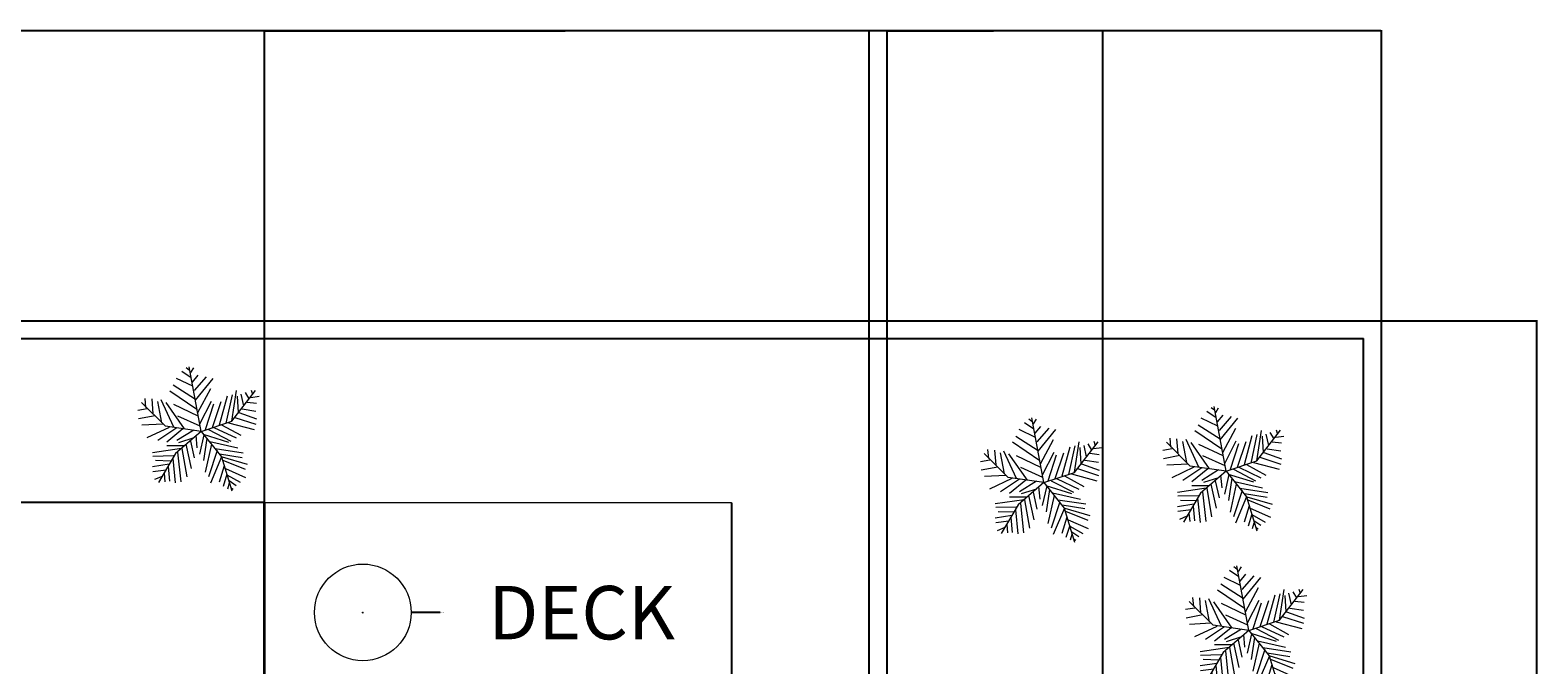
# Model space of a CAD drawing. Units: inches. Extents: x -86 to 773, y -188 to 560.
# Tile 6 of 6: x 392 to 773, y 400 to 560. Entities that reach past the tile are written whole.
import ezdxf

# ---------------------------------------------------------------- set-up
doc = ezdxf.new("R2010")
doc.units = ezdxf.units.IN
doc.header["$MEASUREMENT"] = 0
for name, color, linetype, lineweight in [('A-ANNO-DIMS', 2, 'Continuous', 18), ('A-AREA-IDEN', 7, 'Continuous', 25), ('A-FURN', 8, 'Continuous', 18), ('A-WALL', 7, 'Continuous', 35), ('C-PROP', 7, 'Continuous', 25), ('L-HRDS', 7, 'Continuous', 18), ('L-PLNT-TREE', 8, 'Continuous', 9)]:
    doc.layers.add(name, color=color, linetype=linetype, lineweight=lineweight)
doc.styles.get("Standard").update_dxf_attribs({"font": 'arial.ttf'})
doc.dimstyles.get("Standard").update_dxf_attribs({"dimtxt": 0.18, "dimasz": 0.18, "dimexe": 0.18, "dimexo": 0.0625, "dimgap": 0.09, "dimtad": 0, "dimtih": 1, "dimtoh": 1, "dimdec": 4, "dimzin": 0, "dimdsep": 46, "dimtxsty": 'Standard', "dimcen": 0.09, "dimadec": 0, "dimazin": 0, "dimtfac": 1, "dimtdec": 4, "dimtofl": 0, "dimtmove": 0, "dimatfit": 3, "dimfxl": 1, "dimtolj": 1, "dimtzin": 0, "dimarcsym": 0})

# ---------------------------------------------------------------- blocks, each defined once
blk = doc.blocks.new('Trees - Metric')
for p, q in [((-258.7244, 1362.456), (-332.3336, 1421.4348)), ((0, 0), (-266.7, 1447.8)), ((-231.1146, 1315.2628), (-166.7002, 1421.4348)), ((-129.8956, 713.6638), (-626.7704, 1032.1544)), ((-185.1152, 1008.5578), (-553.1612, 1185.4942)), ((-221.9198, 1197.3052), (-433.5526, 1338.8594)), ((-194.31, 1102.9442), (-65.4812, 1256.284)), ((-148.3106, 914.1968), (118.5418, 1220.9018)), ((-129.8956, 701.8528), (265.7602, 1185.4942)), ((-1234.059, 536.7274), (-1252.4486, 737.2604)), ((-1105.2302, 725.4494), (-1077.6458, 395.1732)), ((-902.8176, 713.6638), (-617.5756, 100.2538)), ((-93.091, 489.5342), (-700.3796, 902.3858)), ((-74.7014, 418.7444), (219.7608, 961.39)), ((-28.6766, 171.0436), (228.9556, 678.2816)), ((412.9786, 147.447), (587.8068, 796.2392)), ((560.197, 182.8292), (698.2206, 819.8358)), ((685.8, 228.6), (1219.2, 914.4)), ((689.0258, 230.0224), (790.2448, 914.1968)), ((808.6344, 784.4282), (827.0494, 418.7444)), ((891.4384, 831.6214), (946.658, 572.1096)), ((983.4626, 867.0036), (1066.2666, 725.4494)), ((1112.2914, 760.8316), (1296.3144, 784.4282)), ((1121.4862, 925.9824), (1149.0706, 831.6214)), ((-1206.4492, 501.3198), (-1418.082, 465.9376)), ((-1031.621, 347.98), (-1399.667, 277.1902)), ((-800.1, 114.3), (-1333.5, 647.7)), ((-976.4268, 666.4706), (-884.4026, 194.6402)), ((-369.1382, 53.086), (-783.1836, 642.874)), ((-617.5756, 607.4918), (-74.7014, 347.98)), ((-525.5514, 347.98), (-28.6766, 123.8504)), ((100.1268, 41.275), (284.1498, 619.2774)), ((256.5654, 88.4682), (449.7832, 666.4706)), ((845.439, 418.7444), (1241.0948, 277.1902)), ((919.0482, 501.3198), (1222.6798, 454.152)), ((1029.462, 654.685), (1241.0948, 631.0884)), ((-847.598, 159.2326), (-1326.0578, 135.636)), ((-718.7946, 88.4682), (-1215.644, -147.447)), ((-543.9664, 76.6572), (-967.2066, -206.4512)), ((0, 0), (-800.1, 114.3)), ((-405.9428, 53.086), (-764.794, -241.8334)), ((0, 0), (-571.5, -495.3)), ((-166.7002, 29.4894), (-543.9664, -206.4512)), ((0, 0), (685.8, 228.6)), ((0, 0), (457.2, -571.5)), ((164.5412, 41.275), (661.416, -218.2368)), ((284.1498, 88.4682), (781.0246, -147.447)), ((458.978, 147.447), (891.4384, -88.4682)), ((615.4166, 194.6402), (1185.8752, 41.275)), ((753.4148, 312.5978), (1222.6798, 159.2326)), ((-387.5278, -324.4088), (-764.794, -324.4088)), ((-166.7002, -147.447), (-507.1618, -253.619)), ((-341.5284, -289.0012), (-221.9198, -831.6214)), ((-240.3094, -218.2368), (-157.5054, -595.7062)), ((-120.7008, -88.4682), (-93.091, -371.5766)), ((63.3222, -76.6826), (-37.8714, -513.1308)), ((44.9326, -64.897), (615.4166, -241.8334)), ((127.7366, -159.258), (54.1274, -654.685)), ((228.9556, -289.0012), (90.932, -914.1968)), ((192.151, -230.0224), (817.8292, -371.5766)), ((-442.7474, -383.3876), (-1086.8406, -477.7486)), ((-617.5756, -548.5384), (-1077.6458, -560.324)), ((-681.9646, -666.496), (-1022.4262, -654.685)), ((-571.5, -495.3), (-952.5, -1143)), ((-635.9652, -607.5172), (-580.771, -1150.1374)), ((-525.5514, -465.963), (-451.9422, -1126.5408)), ((-433.5526, -383.3876), (-323.1134, -1020.3688)), ((357.759, -430.5554), (164.5412, -1020.3688)), ((458.978, -572.1096), (210.5406, -1161.923)), ((311.7596, -383.3876), (937.4378, -477.7486)), ((412.9786, -501.3452), (919.0482, -583.9206)), ((457.2, -571.5), (685.8, -1333.5)), ((468.1982, -572.1096), (1029.462, -737.2604)), ((486.5878, -642.8994), (983.4626, -843.4324)), ((-718.7946, -737.2604), (-1086.8406, -796.2392)), ((-783.1836, -867.029), (-1077.6458, -902.4112)), ((-875.2078, -1008.5832), (-1040.8412, -1079.3476)), ((-829.2084, -937.7934), (-810.7934, -1126.5408)), ((-737.1842, -784.4536), (-709.5744, -1114.7298)), ((514.1976, -772.6426), (403.7838, -1138.3264)), ((578.612, -961.39), (495.7826, -1232.7128)), ((541.8074, -831.6214), (992.6574, -1032.1544)), ((578.612, -973.1756), (873.0488, -1138.3264)), ((624.6114, -1161.923), (587.8068, -1291.6916)), ((624.6114, -1102.9442), (781.0246, -1209.1162)), ((679.8056, -1268.095), (716.6102, -1291.6916))]:
    blk.add_line(p, q)
blk = doc.blocks.new('*D45')
at = {"layer": 'A-ANNO-DIMS', "color": 0, "lineweight": -2, "transparency": 16777216}
for p, q in [((-46.55, 486.72), (-46.55, 560.19)), ((-46.37, 560.01), (343.16, 560.01)), ((733.27, 560.01), (343.74, 560.01)), ((733.45, 486.72), (733.45, 560.19))]:
    blk.add_line(p, q, dxfattribs=at)
at = {"layer": 'A-ANNO-DIMS', "color": 0, "transparency": 16777216}
for points in [[(-46.37, 560.04), (-46.37, 559.98), (-46.55, 560.01)], [(733.27, 560.04), (733.27, 559.98), (733.45, 560.01)]]:
    blk.add_solid(points, dxfattribs=at)
at = {"layer": 'Defpoints', "color": 0, "transparency": 16777216}
for p in [(733.45, 560.01), (-46.55, 486.66), (733.45, 486.66)]:
    blk.add_point(p, dxfattribs=at)
at = {"layer": 'A-ANNO-DIMS', "color": 0, "transparency": 16777216, "insert": (343.45, 560.01), "char_height": 0.18, "attachment_point": 5}
blk.add_mtext('\\A1;780', dxfattribs=at)
blk = doc.blocks.new('*D46')
at = {"layer": 'A-ANNO-DIMS', "color": 0, "lineweight": -2, "transparency": 16777216}
for p, q in [((733.51, 486.66), (772.88, 486.66)), ((772.7, 486.48), (772.7, 169.55)), ((772.7, -147.74), (772.7, 169.19)), ((733.51, -147.92), (772.88, -147.92))]:
    blk.add_line(p, q, dxfattribs=at)
at = {"layer": 'A-ANNO-DIMS', "color": 0, "transparency": 16777216}
for points in [[(772.67, 486.48), (772.73, 486.48), (772.7, 486.66)], [(772.67, -147.74), (772.73, -147.74), (772.7, -147.92)]]:
    blk.add_solid(points, dxfattribs=at)
at = {"layer": 'Defpoints', "color": 0, "transparency": 16777216}
for p in [(733.45, 486.66), (772.7, 486.66), (733.45, -147.92)]:
    blk.add_point(p, dxfattribs=at)
at = {"layer": 'A-ANNO-DIMS', "color": 0, "transparency": 16777216, "insert": (772.7, 169.37), "char_height": 0.18, "attachment_point": 5}
blk.add_mtext('\\A1;634.6', dxfattribs=at)
blk = doc.blocks.new('*D54')
at = {"layer": 'A-ANNO-DIMS', "color": 0, "lineweight": -2, "transparency": 16777216}
for p, q in [((451.03, 440.67), (451.03, -187.76)), ((569.11, 440.67), (569.11, -187.76)), ((451.21, -187.58), (509.62, -187.58)), ((568.93, -187.58), (510.53, -187.58))]:
    blk.add_line(p, q, dxfattribs=at)
at = {"layer": 'A-ANNO-DIMS', "color": 0, "transparency": 16777216}
for points in [[(451.21, -187.55), (451.21, -187.61), (451.03, -187.58)], [(568.93, -187.55), (568.93, -187.61), (569.11, -187.58)]]:
    blk.add_solid(points, dxfattribs=at)
at = {"layer": 'Defpoints', "color": 0, "transparency": 16777216}
for p in [(451.03, 440.74), (569.11, 440.74), (569.11, -187.58)]:
    blk.add_point(p, dxfattribs=at)
at = {"layer": 'A-ANNO-DIMS', "color": 0, "transparency": 16777216, "insert": (510.07, -187.58), "char_height": 0.18, "attachment_point": 5}
blk.add_mtext('\\A1;118.08', dxfattribs=at)
blk = doc.blocks.new('*D55')
at = {"layer": 'A-ANNO-DIMS', "color": 0, "lineweight": -2, "transparency": 16777216}
for p, q in [((450.97, 440.74), (-85.98, 440.74)), ((-85.8, 440.56), (-85.8, 403.81)), ((-85.8, 366.7), (-85.8, 403.45)), ((450.97, 366.52), (-85.98, 366.52))]:
    blk.add_line(p, q, dxfattribs=at)
at = {"layer": 'A-ANNO-DIMS', "color": 0, "transparency": 16777216}
for points in [[(-85.83, 440.56), (-85.77, 440.56), (-85.8, 440.74)], [(-85.83, 366.7), (-85.77, 366.7), (-85.8, 366.52)]]:
    blk.add_solid(points, dxfattribs=at)
at = {"layer": 'Defpoints', "color": 0, "transparency": 16777216}
for p in [(451.03, 440.74), (-85.8, 366.52), (451.03, 366.52)]:
    blk.add_point(p, dxfattribs=at)
at = {"layer": 'A-ANNO-DIMS', "color": 0, "transparency": 16777216, "insert": (-85.8, 403.63), "char_height": 0.18, "attachment_point": 5}
blk.add_mtext('\\A1;74.22', dxfattribs=at)
blk = doc.blocks.new('*D67')
at = {"layer": 'A-ANNO-DIMS', "color": 0, "lineweight": -2, "transparency": 16777216}
for p, q in [((451.03, 204.72), (451.03, 560.19)), ((451.21, 560.01), (527.05, 560.01)), ((603.79, 560.01), (527.96, 560.01)), ((603.97, 204.64), (603.97, 560.19))]:
    blk.add_line(p, q, dxfattribs=at)
at = {"layer": 'A-ANNO-DIMS', "color": 0, "transparency": 16777216}
for points in [[(451.21, 560.04), (451.21, 559.98), (451.03, 560.01)], [(603.79, 560.04), (603.79, 559.98), (603.97, 560.01)]]:
    blk.add_solid(points, dxfattribs=at)
at = {"layer": 'Defpoints', "color": 0, "transparency": 16777216}
for p in [(603.97, 560.01), (451.03, 204.65), (603.97, 204.58)]:
    blk.add_point(p, dxfattribs=at)
at = {"layer": 'A-ANNO-DIMS', "color": 0, "transparency": 16777216, "insert": (527.5, 560.01), "char_height": 0.18, "attachment_point": 5}
blk.add_mtext('\\A1;152.94', dxfattribs=at)
blk = doc.blocks.new('*D68')
at = {"layer": 'A-ANNO-DIMS', "color": 0, "lineweight": -2, "transparency": 16777216}
for p, q in [((608.47, 362.08), (608.47, 560.19)), ((608.65, 560.01), (635.35, 560.01)), ((662.83, 560.01), (636.13, 560.01)), ((663.01, 362.08), (663.01, 560.19))]:
    blk.add_line(p, q, dxfattribs=at)
at = {"layer": 'A-ANNO-DIMS', "color": 0, "transparency": 16777216}
for points in [[(608.65, 560.04), (608.65, 559.98), (608.47, 560.01)], [(662.83, 560.04), (662.83, 559.98), (663.01, 560.01)]]:
    blk.add_solid(points, dxfattribs=at)
at = {"layer": 'Defpoints', "color": 0, "transparency": 16777216}
for p in [(663.01, 560.01), (608.47, 362.02), (663.01, 362.02)]:
    blk.add_point(p, dxfattribs=at)
at = {"layer": 'A-ANNO-DIMS', "color": 0, "transparency": 16777216, "insert": (635.74, 560.01), "char_height": 0.18, "attachment_point": 5}
blk.add_mtext('\\A1;54.54', dxfattribs=at)
blk = doc.blocks.new('*D93')
at = {"layer": 'A-ANNO-DIMS', "color": 0, "lineweight": -2, "transparency": 16777216}
for p, q in [((475.82, 412.91), (476, 412.91)), ((475.91, 412.82), (475.91, 413)), ((495.48, 412.91), (488.32, 412.91))]:
    blk.add_line(p, q, dxfattribs=at)
at = {"layer": 'A-ANNO-DIMS', "color": 0, "transparency": 16777216}
blk.add_solid([(488.32, 412.94), (488.32, 412.88), (488.14, 412.91)], dxfattribs=at)
at = {"layer": 'Defpoints', "color": 0, "transparency": 16777216}
for p in [(463.68, 412.91), (488.14, 412.91)]:
    blk.add_point(p, dxfattribs=at)
at = {"layer": 'A-ANNO-DIMS', "color": 0, "transparency": 16777216, "insert": (495.97, 412.91), "char_height": 0.18, "attachment_point": 5}
blk.add_mtext('\\A1;∅24.46', dxfattribs=at)

msp = doc.modelspace()

# ---------------------------------------------------------------- linework, layer by layer
at = {"layer": 'A-FURN'}
msp.add_circle((475.9139, 412.9106), 12.2298, dxfattribs=at)
at = {"layer": 'A-WALL'}
msp.add_line((451.0315, 240.3369), (451.0315, 440.7367), dxfattribs=at)
at = {"layer": 'C-PROP'}
for p, q in [((-46.5485, 486.6589), (733.4515, 486.6589)), ((733.4515, -147.9172), (733.4515, 486.6589)), ((-42.0485, 482.1589), (728.9515, 482.1589)), ((728.9515, -143.4172), (728.9515, 482.1589))]:
    msp.add_line(p, q, dxfattribs=at)
at = {"layer": 'L-HRDS'}
msp.add_line((569.1115, 366.5167), (569.1115, 440.7367), dxfattribs=at)
msp.add_lwpolyline([(451.0315, 440.7367), (569.1115, 440.7367)], dxfattribs=at)

# ---------------------------------------------------------------- block references
at = {"layer": 'L-PLNT-TREE', "xscale": 0.0112992005060107, "yscale": 0.0112992005060107, "zscale": 0.0112992005060107}
for p in [(435.0347, 458.7065), (648.1043, 445.7618), (694.1734, 448.6384), (699.932, 408.366)]:
    msp.add_blockref('Trees - Metric', p, dxfattribs=at)

# ---------------------------------------------------------------- texts
at = {"layer": 'A-AREA-IDEN'}
msp.add_text('DECK', height=13.52574, dxfattribs=at).set_placement((507.6078, 406.0941))

# ---------------------------------------------------------------- dimensions: what is measured, and where the dimension line sits
at = {"layer": 'A-ANNO-DIMS'}
for base, p1, p2, override, picture, middle in [((733.4515, 560.0063), (-46.5485, 486.6589), (733.4515, 486.6589), {"dimdec": 0, "dimlfac": 1, "dimrnd": 0, "dimzin": 0, "dimdsep": 46, "dimlunit": 2}, '*D45', (343.4515, 560.0063)), ((603.9715, 560.0063), (451.0315, 204.6526), (603.9715, 204.5767), {"dimdec": 2, "dimlfac": 1, "dimrnd": 0, "dimzin": 0, "dimdsep": 46, "dimlunit": 2}, '*D67', (527.5015, 560.0063)), ((663.0115, 560.0063), (608.4715, 362.0167), (663.0115, 362.0167), {"dimdec": 2, "dimlfac": 1, "dimrnd": 0, "dimzin": 0, "dimdsep": 46, "dimlunit": 2}, '*D68', (635.7415, 560.0063)), ((569.1115, -187.578), (451.0315, 440.7367), (569.1115, 440.7367), {"dimdec": 2, "dimlfac": 1, "dimrnd": 0, "dimzin": 0, "dimdsep": 46, "dimlunit": 2}, '*D54', (510.0715, -187.578))]:
    dim = msp.add_linear_dim(base=base, p1=p1, p2=p2, dimstyle='Standard', override=override, dxfattribs=at)
    dim.commit()
    dim.dimension.update_dxf_attribs({"geometry": picture, "text_midpoint": middle})
for base, p1, p2, override, picture, middle in [((772.7015, 486.6589), (733.4515, -147.9172), (733.4515, 486.6589), {"dimdec": 1, "dimlfac": 1, "dimrnd": 0, "dimzin": 0, "dimdsep": 46, "dimlunit": 2}, '*D46', (772.7015, 169.3709)), ((-85.7985, 366.5167), (451.0315, 440.7367), (451.0315, 366.5167), {"dimdec": 2, "dimlfac": 1, "dimrnd": 0, "dimzin": 0, "dimdsep": 46, "dimlunit": 2}, '*D55', (-85.7985, 403.6267))]:
    dim = msp.add_linear_dim(base=base, p1=p1, p2=p2, angle=90, dimstyle='Standard', override=override, dxfattribs=at)
    dim.commit()
    dim.dimension.update_dxf_attribs({"geometry": picture, "text_midpoint": middle})
dim = msp.add_diameter_dim_2p(p1=(463.6842, 412.9102), p2=(488.1437, 412.911), dimstyle='Standard', override={"dimdec": 2, "dimlfac": 1, "dimrnd": 0, "dimzin": 0, "dimdsep": 46, "dimlunit": 2}, dxfattribs=at)
dim.commit()
dim.dimension.update_dxf_attribs({"geometry": '*D93', "text_midpoint": (495.4816, 412.9112), "dimtype": 163})

doc.saveas('drawing.dxf')
